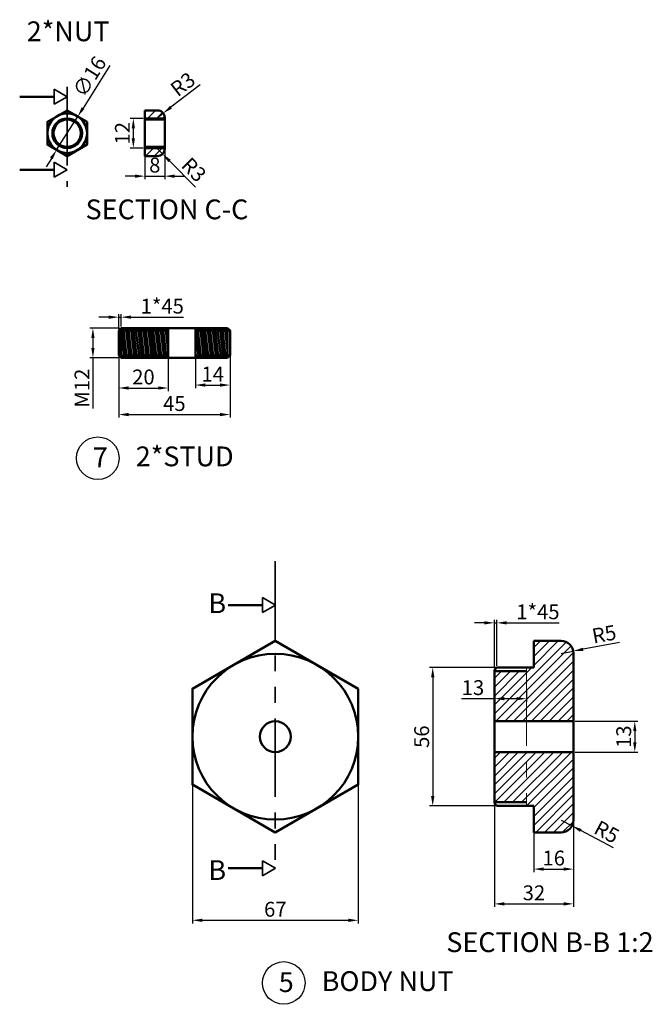
# Model space of a CAD drawing. Units: millimetres. Extents: x 4194 to 4882, y 3816 to 4286.
# Tile 3 of 3: x 4626 to 4882, y 3853 to 4251. Entities that reach past the tile are written whole.
import ezdxf

# ---------------------------------------------------------------- set-up
doc = ezdxf.new("R2010")
doc.units = ezdxf.units.MM
doc.linetypes.add('CENTER', pattern=[50.8, 31.75, -6.35, 6.35, -6.35])
doc.linetypes.add('PHANTOM', pattern=[63.5, 31.75, -6.35, 6.35, -6.35, 6.35, -6.35])
for name, color, linetype, lineweight in [('M-CNTR', 1, 'CENTER', 18), ('M-DIMS', 2, 'Continuous', 25), ('M-HATC', 8, 'Continuous', 18), ('M-OUTL', 7, 'Continuous', 50), ('M-SECT', 6, 'PHANTOM', 35), ('M-TEXT', 3, 'Continuous', 25)]:
    doc.layers.add(name, color=color, linetype=linetype, lineweight=lineweight)
doc.styles.get("Standard").update_dxf_attribs({"font": 'arial.ttf'})
doc.dimstyles.new('ISO-25', dxfattribs={"dimtxt": 6, "dimasz": 4, "dimexe": 1.25, "dimexo": 0.625, "dimtad": 1, "dimdec": 0, "dimtxsty": 'Standard', "dimcen": 2.5, "dimadec": 0, "dimazin": 0, "dimtfac": 1, "dimtdec": 0, "dimtmove": 0, "dimatfit": 3, "dimfxl": 1, "dimarcsym": 0})

# ---------------------------------------------------------------- blocks, each defined once
blk = doc.blocks.new('*D33')
at = {"layer": 'Defpoints', "color": 0, "transparency": 16777216}
for p in [(4649.53, 4211.53), (4640.99, 4198)]:
    blk.add_point(p, dxfattribs=at)
at = {"layer": 'M-DIMS', "color": 0, "lineweight": -2, "transparency": 16777216}
for p, q in [((4662.55, 4232.13), (4651.67, 4214.91)), ((4640.99, 4198), (4649.53, 4211.53)), ((4638.85, 4194.62), (4636.72, 4191.24))]:
    blk.add_line(p, q, dxfattribs=at)
at = {"layer": 'M-DIMS', "color": 0, "transparency": 16777216}
for points in [[(4651.11, 4215.27), (4652.23, 4214.55), (4649.53, 4211.53)], [(4638.29, 4194.97), (4639.42, 4194.26), (4640.99, 4198)]]:
    blk.add_solid(points, dxfattribs=at)
at = {"layer": 'M-DIMS', "color": 0, "transparency": 16777216, "insert": (4654.92, 4227.27), "char_height": 6, "attachment_point": 5, "rotation": 57.7237}
blk.add_mtext('∅16', dxfattribs=at)
blk = doc.blocks.new('*D35')
at = {"layer": 'Defpoints', "color": 0, "transparency": 16777216}
for p in [(4676.65, 4210.76), (4671.98, 4198.76), (4676.65, 4198.76)]:
    blk.add_point(p, dxfattribs=at)
at = {"layer": 'M-DIMS', "color": 0, "lineweight": -2, "transparency": 16777216}
for p, q in [((4676.02, 4210.76), (4670.73, 4210.76)), ((4671.98, 4206.76), (4671.98, 4202.76)), ((4676.02, 4198.76), (4670.73, 4198.76))]:
    blk.add_line(p, q, dxfattribs=at)
at = {"layer": 'M-DIMS', "color": 0, "transparency": 16777216}
for points in [[(4671.31, 4206.76), (4672.64, 4206.76), (4671.98, 4210.76)], [(4671.31, 4202.76), (4672.64, 4202.76), (4671.98, 4198.76)]]:
    blk.add_solid(points, dxfattribs=at)
at = {"layer": 'M-DIMS', "color": 0, "transparency": 16777216, "insert": (4668.34, 4204.76), "char_height": 6, "attachment_point": 5, "rotation": 90}
blk.add_mtext('12', dxfattribs=at)
blk = doc.blocks.new('*D36')
at = {"layer": 'Defpoints', "color": 0, "transparency": 16777216}
for p in [(4684.65, 4202.03), (4676.65, 4196.66), (4684.65, 4187.42)]:
    blk.add_point(p, dxfattribs=at)
at = {"layer": 'M-DIMS', "color": 0, "lineweight": -2, "transparency": 16777216}
for p, q in [((4684.65, 4201.41), (4684.65, 4186.17)), ((4676.65, 4196.03), (4676.65, 4186.17)), ((4672.65, 4187.42), (4668.65, 4187.42)), ((4676.65, 4187.42), (4684.65, 4187.42)), ((4688.65, 4187.42), (4692.65, 4187.42))]:
    blk.add_line(p, q, dxfattribs=at)
at = {"layer": 'M-DIMS', "color": 0, "transparency": 16777216}
for points in [[(4672.65, 4188.08), (4672.65, 4186.75), (4676.65, 4187.42)], [(4688.65, 4188.08), (4688.65, 4186.75), (4684.65, 4187.42)]]:
    blk.add_solid(points, dxfattribs=at)
at = {"layer": 'M-DIMS', "color": 0, "transparency": 16777216, "insert": (4680.65, 4191.11), "char_height": 6, "attachment_point": 5}
blk.add_mtext('8', dxfattribs=at)
blk = doc.blocks.new('*D37')
at = {"layer": 'Defpoints', "color": 0, "transparency": 16777216}
for p in [(4681.65, 4211), (4684.03, 4212.83)]:
    blk.add_point(p, dxfattribs=at)
at = {"layer": 'M-DIMS', "color": 0, "lineweight": -2, "transparency": 16777216}
for p, q in [((4699.03, 4224.36), (4687.2, 4215.27)), ((4681.65, 4211), (4684.03, 4212.83))]:
    blk.add_line(p, q, dxfattribs=at)
at = {"layer": 'M-DIMS', "color": 0, "transparency": 16777216}
blk.add_solid([(4686.79, 4215.8), (4687.6, 4214.74), (4684.03, 4212.83)], dxfattribs=at)
at = {"layer": 'M-DIMS', "color": 0, "transparency": 16777216, "insert": (4692.45, 4223.96), "char_height": 6, "attachment_point": 5, "rotation": 37.5448}
blk.add_mtext('R3', dxfattribs=at)
blk = doc.blocks.new('*D38')
at = {"layer": 'Defpoints', "color": 0, "transparency": 16777216}
for p in [(4666.06, 4114.99), (4686.06, 4114.99), (4686.06, 4101.8)]:
    blk.add_point(p, dxfattribs=at)
at = {"layer": 'M-DIMS', "color": 0, "lineweight": -2, "transparency": 16777216}
for p, q in [((4666.06, 4114.36), (4666.06, 4100.55)), ((4686.06, 4114.36), (4686.06, 4100.55)), ((4670.06, 4101.8), (4682.06, 4101.8))]:
    blk.add_line(p, q, dxfattribs=at)
at = {"layer": 'M-DIMS', "color": 0, "transparency": 16777216}
for points in [[(4670.06, 4102.47), (4670.06, 4101.14), (4666.06, 4101.8)], [(4682.06, 4102.47), (4682.06, 4101.14), (4686.06, 4101.8)]]:
    blk.add_solid(points, dxfattribs=at)
at = {"layer": 'M-DIMS', "color": 0, "transparency": 16777216, "insert": (4676.06, 4105.49), "char_height": 6, "attachment_point": 5}
blk.add_mtext('20', dxfattribs=at)
blk = doc.blocks.new('*D39')
at = {"layer": 'Defpoints', "color": 0, "transparency": 16777216}
for p in [(4697.06, 4117.22), (4711.06, 4117.22), (4711.06, 4102.99)]:
    blk.add_point(p, dxfattribs=at)
at = {"layer": 'M-DIMS', "color": 0, "lineweight": -2, "transparency": 16777216}
for p, q in [((4697.06, 4116.6), (4697.06, 4101.74)), ((4711.06, 4116.6), (4711.06, 4101.74)), ((4701.06, 4102.99), (4707.06, 4102.99))]:
    blk.add_line(p, q, dxfattribs=at)
at = {"layer": 'M-DIMS', "color": 0, "transparency": 16777216}
for points in [[(4701.06, 4103.66), (4701.06, 4102.33), (4697.06, 4102.99)], [(4707.06, 4103.66), (4707.06, 4102.33), (4711.06, 4102.99)]]:
    blk.add_solid(points, dxfattribs=at)
at = {"layer": 'M-DIMS', "color": 0, "transparency": 16777216, "insert": (4704.06, 4106.63), "char_height": 6, "attachment_point": 5}
blk.add_mtext('14', dxfattribs=at)
blk = doc.blocks.new('*D40')
at = {"layer": 'Defpoints', "color": 0, "transparency": 16777216}
for p in [(4666.06, 4119.99), (4711.06, 4118.23), (4711.06, 4091.07)]:
    blk.add_point(p, dxfattribs=at)
at = {"layer": 'M-DIMS', "color": 0, "lineweight": -2, "transparency": 16777216}
for p, q in [((4666.06, 4119.36), (4666.06, 4089.82)), ((4711.06, 4117.61), (4711.06, 4089.82)), ((4670.06, 4091.07), (4707.06, 4091.07))]:
    blk.add_line(p, q, dxfattribs=at)
at = {"layer": 'M-DIMS', "color": 0, "transparency": 16777216}
for points in [[(4670.06, 4091.74), (4670.06, 4090.4), (4666.06, 4091.07)], [(4707.06, 4091.74), (4707.06, 4090.4), (4711.06, 4091.07)]]:
    blk.add_solid(points, dxfattribs=at)
at = {"layer": 'M-DIMS', "color": 0, "transparency": 16777216, "insert": (4688.56, 4094.75), "char_height": 6, "attachment_point": 5}
blk.add_mtext('45', dxfattribs=at)
blk = doc.blocks.new('*D41')
at = {"layer": 'Defpoints', "color": 0, "transparency": 16777216}
for p in [(4667.06, 4130.43), (4666.06, 4124.99), (4667.06, 4125.99)]:
    blk.add_point(p, dxfattribs=at)
at = {"layer": 'M-DIMS', "color": 0, "lineweight": -2, "transparency": 16777216}
for p, q in [((4662.06, 4130.43), (4658.06, 4130.43)), ((4666.06, 4125.61), (4666.06, 4131.68)), ((4666.06, 4130.43), (4667.06, 4130.43)), ((4667.06, 4126.61), (4667.06, 4131.68)), ((4671.06, 4130.43), (4692.31, 4130.43))]:
    blk.add_line(p, q, dxfattribs=at)
at = {"layer": 'M-DIMS', "color": 0, "transparency": 16777216}
for points in [[(4662.06, 4131.1), (4662.06, 4129.77), (4666.06, 4130.43)], [(4671.06, 4131.1), (4671.06, 4129.77), (4667.06, 4130.43)]]:
    blk.add_solid(points, dxfattribs=at)
at = {"layer": 'M-DIMS', "color": 0, "transparency": 16777216, "insert": (4683.68, 4134.12), "char_height": 6, "attachment_point": 5}
blk.add_mtext('1*45', dxfattribs=at)
blk = doc.blocks.new('*D42')
at = {"layer": 'Defpoints', "color": 0, "transparency": 16777216}
for p in [(4667.06, 4125.99), (4655.64, 4113.99), (4667.06, 4113.99)]:
    blk.add_point(p, dxfattribs=at)
at = {"layer": 'M-DIMS', "color": 0, "lineweight": -2, "transparency": 16777216}
for p, q in [((4666.43, 4125.99), (4654.39, 4125.99)), ((4655.64, 4121.99), (4655.64, 4117.99)), ((4666.43, 4113.99), (4654.39, 4113.99)), ((4655.64, 4113.99), (4655.64, 4093.5))]:
    blk.add_line(p, q, dxfattribs=at)
at = {"layer": 'M-DIMS', "color": 0, "transparency": 16777216}
for points in [[(4654.98, 4121.99), (4656.31, 4121.99), (4655.64, 4125.99)], [(4654.98, 4117.99), (4656.31, 4117.99), (4655.64, 4113.99)]]:
    blk.add_solid(points, dxfattribs=at)
at = {"layer": 'M-DIMS', "color": 0, "transparency": 16777216, "insert": (4652.01, 4101.74), "char_height": 6, "attachment_point": 5, "rotation": 90}
blk.add_mtext('M12', dxfattribs=at)
blk = doc.blocks.new('*D43')
at = {"layer": 'Defpoints', "color": 0, "transparency": 16777216}
for p in [(4695.85, 3960.89), (4762.85, 3960.89), (4762.85, 3886.69)]:
    blk.add_point(p, dxfattribs=at)
at = {"layer": 'M-DIMS', "color": 0, "lineweight": -2, "transparency": 16777216}
for p, q in [((4695.85, 3960.27), (4695.85, 3885.44)), ((4762.85, 3960.27), (4762.85, 3885.44)), ((4699.85, 3886.69), (4758.85, 3886.69))]:
    blk.add_line(p, q, dxfattribs=at)
at = {"layer": 'M-DIMS', "color": 0, "transparency": 16777216}
for points in [[(4699.85, 3887.35), (4699.85, 3886.02), (4695.85, 3886.69)], [(4758.85, 3887.35), (4758.85, 3886.02), (4762.85, 3886.69)]]:
    blk.add_solid(points, dxfattribs=at)
at = {"layer": 'M-DIMS', "color": 0, "transparency": 16777216, "insert": (4729.35, 3890.37), "char_height": 6, "attachment_point": 5}
blk.add_mtext('67', dxfattribs=at)
blk = doc.blocks.new('*D44')
at = {"layer": 'Defpoints', "color": 0, "transparency": 16777216}
for p in [(4833.86, 3925.96), (4849.86, 3927.21), (4849.86, 3907.38)]:
    blk.add_point(p, dxfattribs=at)
at = {"layer": 'M-DIMS', "color": 0, "lineweight": -2, "transparency": 16777216}
for p, q in [((4833.86, 3925.33), (4833.86, 3906.13)), ((4849.86, 3926.58), (4849.86, 3906.13)), ((4837.86, 3907.38), (4845.86, 3907.38))]:
    blk.add_line(p, q, dxfattribs=at)
at = {"layer": 'M-DIMS', "color": 0, "transparency": 16777216}
for points in [[(4837.86, 3908.05), (4837.86, 3906.71), (4833.86, 3907.38)], [(4845.86, 3908.05), (4845.86, 3906.71), (4849.86, 3907.38)]]:
    blk.add_solid(points, dxfattribs=at)
at = {"layer": 'M-DIMS', "color": 0, "transparency": 16777216, "insert": (4841.86, 3911.07), "char_height": 6, "attachment_point": 5}
blk.add_mtext('16', dxfattribs=at)
blk = doc.blocks.new('*D45')
at = {"layer": 'Defpoints', "color": 0, "transparency": 16777216}
for p in [(4817.86, 3944.88), (4849.86, 3944.05), (4849.86, 3893.32)]:
    blk.add_point(p, dxfattribs=at)
at = {"layer": 'M-DIMS', "color": 0, "lineweight": -2, "transparency": 16777216}
for p, q in [((4817.86, 3944.25), (4817.86, 3892.07)), ((4849.86, 3943.43), (4849.86, 3892.07)), ((4821.86, 3893.32), (4845.86, 3893.32))]:
    blk.add_line(p, q, dxfattribs=at)
at = {"layer": 'M-DIMS', "color": 0, "transparency": 16777216}
for points in [[(4821.86, 3893.98), (4821.86, 3892.65), (4817.86, 3893.32)], [(4845.86, 3893.98), (4845.86, 3892.65), (4849.86, 3893.32)]]:
    blk.add_solid(points, dxfattribs=at)
at = {"layer": 'M-DIMS', "color": 0, "transparency": 16777216, "insert": (4833.86, 3897.01), "char_height": 6, "attachment_point": 5}
blk.add_mtext('32', dxfattribs=at)
blk = doc.blocks.new('*D46')
at = {"layer": 'Defpoints', "color": 0, "transparency": 16777216}
for p in [(4818.86, 4006.89), (4817.86, 3987.89), (4818.86, 3988.89)]:
    blk.add_point(p, dxfattribs=at)
at = {"layer": 'M-DIMS', "color": 0, "lineweight": -2, "transparency": 16777216}
for p, q in [((4817.86, 3988.52), (4817.86, 4008.14)), ((4818.86, 3989.52), (4818.86, 4008.14)), ((4813.86, 4006.89), (4809.86, 4006.89)), ((4817.86, 4006.89), (4818.86, 4006.89)), ((4822.86, 4006.89), (4844.11, 4006.89))]:
    blk.add_line(p, q, dxfattribs=at)
at = {"layer": 'M-DIMS', "color": 0, "transparency": 16777216}
for points in [[(4813.86, 4007.56), (4813.86, 4006.23), (4817.86, 4006.89)], [(4822.86, 4007.56), (4822.86, 4006.23), (4818.86, 4006.89)]]:
    blk.add_solid(points, dxfattribs=at)
at = {"layer": 'M-DIMS', "color": 0, "transparency": 16777216, "insert": (4835.49, 4010.58), "char_height": 6, "attachment_point": 5}
blk.add_mtext('1*45', dxfattribs=at)
blk = doc.blocks.new('*D47')
at = {"layer": 'Defpoints', "color": 0, "transparency": 16777216}
for p in [(4825.21, 3988.89), (4792.96, 3932.89), (4824.11, 3932.89)]:
    blk.add_point(p, dxfattribs=at)
at = {"layer": 'M-DIMS', "color": 0, "lineweight": -2, "transparency": 16777216}
for p, q in [((4824.59, 3988.89), (4791.71, 3988.89)), ((4792.96, 3984.89), (4792.96, 3936.89)), ((4823.49, 3932.89), (4791.71, 3932.89))]:
    blk.add_line(p, q, dxfattribs=at)
at = {"layer": 'M-DIMS', "color": 0, "transparency": 16777216}
for points in [[(4792.3, 3984.89), (4793.63, 3984.89), (4792.96, 3988.89)], [(4792.3, 3936.89), (4793.63, 3936.89), (4792.96, 3932.89)]]:
    blk.add_solid(points, dxfattribs=at)
at = {"layer": 'M-DIMS', "color": 0, "transparency": 16777216, "insert": (4789.27, 3960.89), "char_height": 6, "attachment_point": 5, "rotation": 90}
blk.add_mtext('56', dxfattribs=at)
blk = doc.blocks.new('*D48')
at = {"layer": 'Defpoints', "color": 0, "transparency": 16777216}
for p in [(4849.78, 3995.49), (4844.86, 3994.57)]:
    blk.add_point(p, dxfattribs=at)
at = {"layer": 'M-DIMS', "color": 0, "lineweight": -2, "transparency": 16777216}
for p, q in [((4844.86, 3994.57), (4849.78, 3995.49)), ((4868.43, 3998.96), (4853.71, 3996.22))]:
    blk.add_line(p, q, dxfattribs=at)
at = {"layer": 'M-DIMS', "color": 0, "transparency": 16777216}
blk.add_solid([(4853.59, 3996.87), (4853.83, 3995.56), (4849.78, 3995.49)], dxfattribs=at)
at = {"layer": 'M-DIMS', "color": 0, "transparency": 16777216, "insert": (4862.36, 4001.57), "char_height": 6, "attachment_point": 5, "rotation": 10.5295}
blk.add_mtext('R5', dxfattribs=at)
blk = doc.blocks.new('*D49')
at = {"layer": 'Defpoints', "color": 0, "transparency": 16777216}
for p in [(4830.86, 3980.23), (4817.86, 3979.09), (4817.86, 3976.25)]:
    blk.add_point(p, dxfattribs=at)
at = {"layer": 'M-DIMS', "color": 0, "lineweight": -2, "transparency": 16777216}
for p, q in [((4830.86, 3979.61), (4830.86, 3975)), ((4817.86, 3976.25), (4804.58, 3976.25)), ((4817.86, 3978.47), (4817.86, 3975)), ((4826.86, 3976.25), (4821.86, 3976.25))]:
    blk.add_line(p, q, dxfattribs=at)
at = {"layer": 'M-DIMS', "color": 0, "transparency": 16777216}
for points in [[(4821.86, 3976.92), (4821.86, 3975.58), (4817.86, 3976.25)], [(4826.86, 3976.92), (4826.86, 3975.58), (4830.86, 3976.25)]]:
    blk.add_solid(points, dxfattribs=at)
at = {"layer": 'M-DIMS', "color": 0, "transparency": 16777216, "insert": (4809.22, 3979.94), "char_height": 6, "attachment_point": 5}
blk.add_mtext('13', dxfattribs=at)
blk = doc.blocks.new('*D50')
at = {"layer": 'Defpoints', "color": 0, "transparency": 16777216}
for p in [(4849.86, 3967.14), (4849.86, 3954.64), (4874.61, 3954.64)]:
    blk.add_point(p, dxfattribs=at)
at = {"layer": 'M-DIMS', "color": 0, "lineweight": -2, "transparency": 16777216}
for p, q in [((4850.49, 3967.14), (4875.86, 3967.14)), ((4874.61, 3963.14), (4874.61, 3958.64)), ((4850.49, 3954.64), (4875.86, 3954.64))]:
    blk.add_line(p, q, dxfattribs=at)
at = {"layer": 'M-DIMS', "color": 0, "transparency": 16777216}
for points in [[(4873.95, 3963.14), (4875.28, 3963.14), (4874.61, 3967.14)], [(4873.95, 3958.64), (4875.28, 3958.64), (4874.61, 3954.64)]]:
    blk.add_solid(points, dxfattribs=at)
at = {"layer": 'M-DIMS', "color": 0, "transparency": 16777216, "insert": (4870.92, 3960.89), "char_height": 6, "attachment_point": 5, "rotation": 90}
blk.add_mtext('13', dxfattribs=at)
blk = doc.blocks.new('SECTION-ARROW')
for p, q in [((3.04, 5.26), (0, 0)), ((3.04, 5.26), (6.07, 0)), ((6.07, 0), (0, 0))]:
    blk.add_line(p, q)
blk = doc.blocks.new('*D55')
at = {"layer": 'Defpoints', "color": 0, "transparency": 16777216}
for p in [(4681.65, 4198.53), (4683.77, 4196.4)]:
    blk.add_point(p, dxfattribs=at)
at = {"layer": 'M-DIMS', "color": 0, "lineweight": -2, "transparency": 16777216}
for p, q in [((4681.65, 4198.53), (4683.77, 4196.4)), ((4697.15, 4183.02), (4686.6, 4193.58))]:
    blk.add_line(p, q, dxfattribs=at)
at = {"layer": 'M-DIMS', "color": 0, "transparency": 16777216}
blk.add_solid([(4687.07, 4194.05), (4686.13, 4193.1), (4683.77, 4196.4)], dxfattribs=at)
at = {"layer": 'M-DIMS', "color": 0, "transparency": 16777216, "insert": (4695.9, 4189.49), "char_height": 6, "attachment_point": 5, "rotation": 315}
blk.add_mtext('R3', dxfattribs=at)
blk = doc.blocks.new('*D56')
at = {"layer": 'Defpoints', "color": 0, "transparency": 16777216}
for p in [(4844.86, 3927.21), (4849.27, 3924.85)]:
    blk.add_point(p, dxfattribs=at)
at = {"layer": 'M-DIMS', "color": 0, "lineweight": -2, "transparency": 16777216}
for p, q in [((4844.86, 3927.21), (4849.27, 3924.85)), ((4866.01, 3915.92), (4852.8, 3922.97))]:
    blk.add_line(p, q, dxfattribs=at)
at = {"layer": 'M-DIMS', "color": 0, "transparency": 16777216}
blk.add_solid([(4853.12, 3923.56), (4852.49, 3922.38), (4849.27, 3924.85)], dxfattribs=at)
at = {"layer": 'M-DIMS', "color": 0, "transparency": 16777216, "insert": (4862.9, 3921.74), "char_height": 6, "attachment_point": 5, "rotation": 331.8902}
blk.add_mtext('R5', dxfattribs=at)

msp = doc.modelspace()

# ---------------------------------------------------------------- hatches: boundary and pattern name
at = {"layer": 'M-HATC'}
h = msp.add_hatch(dxfattribs=at)
h.set_pattern_fill('ANSI31', color=256, scale=0.8)
h.paths.add_polyline_path([(4681.6471, 4214.0011), (4676.6471, 4214.0011), (4676.6471, 4210.7635), (4684.6471, 4210.7635), (4684.6471, 4211.0011, 0.41421356)])
h.paths.add_polyline_path([(4684.6471, 4198.5259), (4684.6471, 4198.7635), (4676.6471, 4198.7635), (4676.6471, 4195.5259), (4681.6471, 4195.5259, 0.41421356)])
h = msp.add_hatch(dxfattribs=at)
h.set_pattern_fill('ANSI31', color=256, scale=0.8)
h.paths.add_polyline_path([(4849.8629, 3994.5749, 0.41421356), (4844.8629, 3999.5749), (4833.8629, 3999.5749), (4833.8629, 3988.8924), (4830.8629, 3988.8924), (4830.8629, 3967.1424), (4849.8629, 3967.1424)])
h.paths.add_polyline_path([(4830.8629, 3987.3924), (4817.8629, 3987.3924), (4817.8629, 3967.1424), (4830.8629, 3967.1424)])
h.paths.add_polyline_path([(4830.8629, 3954.6424), (4817.8629, 3954.6424), (4817.8629, 3934.3924), (4830.8629, 3934.3924)])
h.paths.add_polyline_path([(4849.8629, 3954.6424), (4830.8629, 3954.6424), (4830.8629, 3934.3924), (4830.8629, 3932.8924), (4833.8629, 3932.8924), (4833.8629, 3922.2099), (4844.8629, 3922.2099, 0.41421356), (4849.8629, 3927.2099)])

# ---------------------------------------------------------------- linework, layer by layer
at = {"layer": 'M-CNTR'}
msp.add_line((4830.8629, 3988.8924), (4830.8629, 3932.8924), dxfattribs=at)
at = {"layer": 'M-OUTL'}
for p, q in [((4640.0046, 4219.4976), (4626.0624, 4219.4976)), ((4676.6471, 4214.0011), (4676.6471, 4195.5259)), ((4681.6471, 4214.0011), (4676.6471, 4214.0011)), ((4676.6471, 4210.7635), (4684.6471, 4210.7635)), ((4676.6471, 4210.2635), (4684.6471, 4210.2635)), ((4684.6471, 4198.5259), (4684.6471, 4211.0011)), ((4676.6471, 4199.2635), (4684.6471, 4199.2635)), ((4676.6471, 4198.7635), (4684.6471, 4198.7635)), ((4676.6471, 4195.5259), (4681.6471, 4195.5259)), ((4640.0046, 4190.0295), (4626.0624, 4190.0295)), ((4666.0592, 4124.9886), (4667.0592, 4125.9886)), ((4666.0592, 4114.9886), (4666.0592, 4124.9886)), ((4666.0592, 4124.9886), (4686.0592, 4124.9886)), ((4667.0592, 4125.9886), (4710.0592, 4125.9886)), ((4667.0592, 4125.9886), (4667.0592, 4113.9886)), ((4667.0592, 4124.9886), (4668.2763, 4114.9886)), ((4668.0592, 4124.9886), (4669.2763, 4114.9886)), ((4669.0592, 4124.9886), (4670.2763, 4114.9886)), ((4670.0592, 4124.9886), (4671.2763, 4114.9886)), ((4671.0592, 4124.9886), (4672.2763, 4114.9886)), ((4672.0592, 4124.9886), (4673.2763, 4114.9886)), ((4673.0592, 4124.9886), (4674.2763, 4114.9886)), ((4674.0592, 4124.9886), (4675.2763, 4114.9886)), ((4675.0592, 4124.9886), (4676.2763, 4114.9886)), ((4676.0592, 4124.9886), (4677.2763, 4114.9886)), ((4677.0592, 4124.9886), (4678.2763, 4114.9886)), ((4678.0592, 4124.9886), (4679.2763, 4114.9886)), ((4679.0592, 4124.9886), (4680.2763, 4114.9886)), ((4680.0592, 4124.9886), (4681.2763, 4114.9886)), ((4681.0592, 4124.9886), (4682.2763, 4114.9886)), ((4682.0592, 4124.9886), (4683.2763, 4114.9886)), ((4683.0592, 4124.9886), (4684.2763, 4114.9886)), ((4684.0592, 4124.9886), (4685.2763, 4114.9886)), ((4685.0592, 4124.9886), (4686.0592, 4116.7719)), ((4686.0592, 4113.9886), (4686.0592, 4125.9886)), ((4697.0592, 4125.9886), (4697.0592, 4113.9886)), ((4697.0592, 4124.9886), (4711.0592, 4124.9886)), ((4697.0592, 4124.9886), (4698.2763, 4114.9886)), ((4698.0592, 4124.9886), (4699.2763, 4114.9886)), ((4699.0592, 4124.9886), (4700.2763, 4114.9886)), ((4700.0592, 4124.9886), (4701.2763, 4114.9886)), ((4701.0592, 4124.9886), (4702.2763, 4114.9886)), ((4702.0592, 4124.9886), (4703.2763, 4114.9886)), ((4703.0592, 4124.9886), (4704.2763, 4114.9886)), ((4704.0592, 4124.9886), (4705.2763, 4114.9886)), ((4705.0592, 4124.9886), (4706.2763, 4114.9886)), ((4706.0592, 4124.9886), (4707.2763, 4114.9886)), ((4707.0592, 4124.9886), (4708.2763, 4114.9886)), ((4708.0592, 4124.9886), (4709.2763, 4114.9886)), ((4709.0592, 4124.9886), (4710.0592, 4116.7719)), ((4710.0592, 4125.9886), (4711.0592, 4124.9886)), ((4710.0592, 4125.9886), (4710.0592, 4113.9886)), ((4711.0592, 4124.9886), (4711.0592, 4114.9886)), ((4666.0592, 4114.9886), (4667.0592, 4113.9886)), ((4686.0592, 4114.9886), (4666.0592, 4114.9886)), ((4711.0592, 4114.9886), (4697.0592, 4114.9886)), ((4711.0592, 4114.9886), (4710.0592, 4113.9886)), ((4710.0592, 4113.9886), (4667.0592, 4113.9886)), ((4724.1866, 4014.0508), (4710.2445, 4014.0508)), ((4833.8629, 3999.5749), (4833.8629, 3988.8924)), ((4833.8629, 3999.5749), (4844.8629, 3999.5749)), ((4849.8629, 3994.5749), (4849.8629, 3960.8924)), ((4817.8629, 3987.8924), (4818.8629, 3988.8924)), ((4817.8629, 3987.8924), (4817.8629, 3960.8924)), ((4817.8629, 3987.3924), (4830.8629, 3987.3924)), ((4818.8629, 3988.8924), (4833.8629, 3988.8924)), ((4762.2572, 3967.1424), (4762.8454, 3967.1424)), ((4817.8629, 3967.1424), (4849.8629, 3967.1424)), ((4817.8629, 3933.8924), (4817.8629, 3960.8924)), ((4849.8629, 3927.2099), (4849.8629, 3960.8924)), ((4762.2572, 3954.6424), (4762.8454, 3954.6424)), ((4817.8629, 3954.6424), (4849.8629, 3954.6424)), ((4817.8629, 3934.3924), (4830.8629, 3934.3924)), ((4817.8629, 3933.8924), (4818.8629, 3932.8924)), ((4818.8629, 3932.8924), (4833.8629, 3932.8924)), ((4833.8629, 3922.2099), (4833.8629, 3932.8924)), ((4833.8629, 3922.2099), (4844.8629, 3922.2099)), ((4724.1866, 3907.734), (4710.2445, 3907.734))]:
    msp.add_line(p, q, dxfattribs=at)
for points in [[(4653.2622, 4209.3823), (4645.2622, 4214.0011), (4637.2622, 4209.3823), (4637.2622, 4200.1447), (4645.2622, 4195.5259), (4653.2622, 4200.1447)], [(4762.8454, 3980.2336), (4729.3454, 3999.5749), (4695.8454, 3980.2336), (4695.8454, 3941.5512), (4729.3454, 3922.2099), (4762.8454, 3941.5512)]]:
    msp.add_lwpolyline(points, close=True, dxfattribs=at)
for centre, radius in [((4645.2622, 4204.7635), 8), ((4645.2622, 4204.7635), 6), ((4645.2622, 4204.7635), 5.5), ((4729.3454, 3960.8924), 33.5), ((4729.3454, 3960.8924), 6.25)]:
    msp.add_circle(centre, radius, dxfattribs=at)
for centre, radius, start, end in [((4681.6471, 4211.0011), 3, 0, 90), ((4681.6471, 4198.5259), 3, 270, 0), ((4844.8629, 3994.5749), 5, 0, 90), ((4844.8629, 3927.2099), 5, 270, 0)]:
    msp.add_arc(centre, radius, start, end, dxfattribs=at)
at = {"layer": 'M-SECT'}
for p, q in [((4645.2622, 4223.5204), (4645.2622, 4183.0807)), ((4729.3454, 4031.7835), (4729.3454, 3905.2451))]:
    msp.add_line(p, q, dxfattribs=at)
at = {"layer": 'M-TEXT'}
for centre in [(4657.6016, 4073.422), (4732.7414, 3861.3496)]:
    msp.add_circle(centre, 8.6164, dxfattribs=at)

# ---------------------------------------------------------------- block references
at = {"layer": 'M-SECT'}
for p, rotation in [((4640.0051, 4216.4619), 29.99999999998718), ((4640.0051, 4186.9938), 30.00000000000203), ((4724.1871, 4011.0151), 30.00000000000949), ((4724.1871, 3904.6983), 30.00000000000949)]:
    msp.add_blockref('SECTION-ARROW', p, dxfattribs=dict(at, rotation=rotation))

# ---------------------------------------------------------------- texts
at = {"layer": 'M-TEXT', "char_height": 8}
for s, width, insert, attachment_point in [('2*NUT', 38.884897, (4628.9147, 4249.9636), 1), ('SECTION C-C', 72.30386, (4652.6787, 4177.9908), 1), ('2*STUD', 38.884897, (4672.9531, 4078.1702), 1), ('7', 8, (4655.5995, 4077.7602), 1), ('B', 8, (4702.3091, 4018.8165), 1), ('B', 8, (4702.3091, 3902.9683), 7), ('SECTION B-B 1:2', 117.140838, (4798.4511, 3881.8344), 1), ('5', 8, (4730.7394, 3865.6878), 1), ('BODY NUT', 60.392338, (4748.093, 3866.0978), 1)]:
    msp.add_mtext_dynamic_manual_height_columns(s, width=width, gutter_width=12.5, heights=[0], dxfattribs=dict(at, insert=insert, attachment_point=attachment_point))

# ---------------------------------------------------------------- dimensions: what is measured, and where the dimension line sits
at = {"layer": 'M-DIMS'}
dim = msp.add_diameter_dim_2p(p1=(4640.9902, 4197.9997), p2=(4649.5342, 4211.5274), dimstyle='ISO-25', override={"dimclrd": 0, "dimclre": 0, "dimclrt": 0}, dxfattribs=at)
dim.commit()
dim.dimension.update_dxf_attribs({"geometry": '*D33', "text_midpoint": (4654.9163, 4227.2702)})
for center, mpoint, override, picture, middle in [((4681.6471, 4211.0011), (4684.0257, 4212.8293), {"dimclrd": 0, "dimclre": 0, "dimclrt": 0}, '*D37', (4692.4511, 4223.9593)), ((4681.6471, 4198.5259), (4683.7684, 4196.4046), {"dimdec": 0, "dimlfac": 1, "dimrnd": 0, "dimzin": 0, "dimdsep": 46, "dimlunit": 2}, '*D55', (4695.8975, 4189.4946)), ((4844.8629, 3994.5749), (4849.7787, 3995.4886), {"dimclrd": 0, "dimclre": 0, "dimclrt": 0}, '*D48', (4862.365, 4001.5671)), ((4844.8629, 3927.2099), (4849.2731, 3924.8541), {"dimdec": 0, "dimlfac": 1, "dimrnd": 0, "dimzin": 0, "dimdsep": 46, "dimlunit": 2}, '*D56', (4862.8997, 3921.743))]:
    dim = msp.add_radius_dim(center=center, mpoint=mpoint, dimstyle='ISO-25', override=override, dxfattribs=at)
    dim.commit()
    dim.dimension.update_dxf_attribs({"geometry": picture, "text_midpoint": middle})
for base, p1, p2, picture, middle in [((4671.9783, 4198.7635), (4676.6471, 4210.7635), (4676.6471, 4198.7635), '*D35', (4668.341, 4204.7635)), ((4792.9626, 3932.8924), (4825.211, 3988.8924), (4824.1117, 3932.8924), '*D47', (4789.2742, 3960.8924)), ((4874.6145836811, 3954.6424023471), (4849.8628569281, 3967.1424023471), (4849.8628569281, 3954.6424023471), '*D50', (4870.92409937, 3960.8924023471))]:
    dim = msp.add_linear_dim(base=base, p1=p1, p2=p2, angle=90, dimstyle='ISO-25', override={"dimclrd": 0, "dimclre": 0, "dimclrt": 0}, dxfattribs=at)
    dim.commit()
    dim.dimension.update_dxf_attribs({"geometry": picture, "text_midpoint": middle})
for base, p1, p2, picture, middle in [((4684.6471, 4187.4181), (4676.6471, 4196.6566), (4684.6471, 4202.0317), '*D36', (4680.6471, 4187.4181)), ((4817.8629, 3976.2493), (4830.8629, 3980.2323), (4817.8629, 3979.0921), '*D49', (4809.2229, 3976.2493))]:
    dim = msp.add_linear_dim(base=base, p1=p1, p2=p2, dimstyle='ISO-25', override={"dimclrd": 0, "dimclre": 0, "dimclrt": 0}, dxfattribs=at)
    dim.commit()
    dim.dimension.update_dxf_attribs({"geometry": picture, "text_midpoint": middle, "dimtype": 160})
dim = msp.add_linear_dim(base=(4667.0592, 4130.4328), p1=(4666.0592, 4124.9886), p2=(4667.0592, 4125.9886), text='<>*45', dimstyle='ISO-25', override={"dimclrd": 0, "dimclre": 0, "dimclrt": 0}, dxfattribs=at)
dim.commit()
dim.dimension.update_dxf_attribs({"geometry": '*D41', "text_midpoint": (4683.6836, 4134.1212)})
dim = msp.add_linear_dim(base=(4655.6444, 4113.9886), p1=(4667.0592, 4125.9886), p2=(4667.0592, 4113.9886), angle=90, text='M<>', dimstyle='ISO-25', override={"dimclrd": 0, "dimclre": 0, "dimclrt": 0}, dxfattribs=at)
dim.commit()
dim.dimension.update_dxf_attribs({"geometry": '*D42', "text_midpoint": (4652.0072, 4101.7429)})
for base, p1, p2, picture, middle in [((4711.0592, 4091.0695), (4666.0592, 4119.9886), (4711.0592, 4118.2329), '*D40', (4688.5592, 4094.7456)), ((4686.0592, 4101.8018), (4666.0592, 4114.9886), (4686.0592, 4114.9886), '*D38', (4676.0592, 4105.4902)), ((4711.0592, 4102.9924), (4697.0592, 4117.2208), (4711.0592, 4117.2208), '*D39', (4704.0592, 4106.6297)), ((4762.8454, 3886.686), (4695.8454, 3960.8924), (4762.8454, 3960.8924), '*D43', (4729.3454, 3890.3744)), ((4849.8629, 3893.3153), (4817.8629, 3944.8794), (4849.8629, 3944.0512), '*D45', (4833.8629, 3897.0058)), ((4849.8629, 3907.3802), (4833.8629, 3925.9599), (4849.8629, 3927.2099), '*D44', (4841.8629, 3911.0686))]:
    dim = msp.add_linear_dim(base=base, p1=p1, p2=p2, dimstyle='ISO-25', override={"dimclrd": 0, "dimclre": 0, "dimclrt": 0}, dxfattribs=at)
    dim.commit()
    dim.dimension.update_dxf_attribs({"geometry": picture, "text_midpoint": middle})
dim = msp.add_linear_dim(base=(4818.8629, 4006.8939), p1=(4817.8629, 3987.8924), p2=(4818.8629, 3988.8924), text='<>*45', dimstyle='ISO-25', override={"dimclrd": 0, "dimclre": 0, "dimclrt": 0}, dxfattribs=at)
dim.commit()
dim.dimension.update_dxf_attribs({"geometry": '*D46', "text_midpoint": (4835.4872, 4006.8939), "dimtype": 160})

doc.saveas('drawing.dxf')
